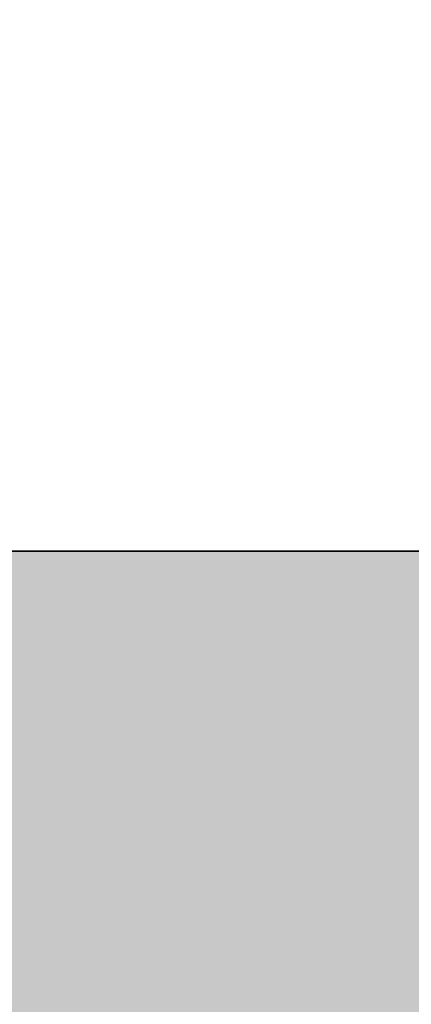
# Model space of a CAD drawing. Units: inches. Extents: x 2696 to 3240, y 1564 to 2310.
# Tile 58 of 76: x 2916.85 to 2921.79, y 2179.88 to 2192.31. Entities that reach past the tile are written whole.
import ezdxf

# ---------------------------------------------------------------- set-up
doc = ezdxf.new("R2010")
doc.units = ezdxf.units.IN
for name, color, linetype, lineweight in [('A-ANNO-DIMS', 3, 'Continuous', 18), ('A-WALL', 7, 'Continuous', 35), ('A-WALL-PATT', 9, 'Continuous', 13)]:
    doc.layers.add(name, color=color, linetype=linetype, lineweight=lineweight)
doc.styles.add('TIMES NEW', font='times.ttf')
doc.dimstyles.new('Siddhuu', dxfattribs={"dimtxt": 6, "dimasz": 2.5, "dimexe": 1.25, "dimexo": 0.625, "dimtad": 1, "dimdec": 1, "dimlunit": 4, "dimtxsty": 'TIMES NEW', "dimcen": 2.5, "dimclrd": 256, "dimclre": 1, "dimclrt": 7, "dimadec": 0, "dimazin": 0, "dimtfac": 1, "dimtdec": 1, "dimtmove": 0, "dimatfit": 3, "dimfxl": 1, "dimtolj": 1, "dimlwd": -1, "dimarcsym": 0})

# ---------------------------------------------------------------- blocks, each defined once
blk = doc.blocks.new('*D59')
at = {"layer": 'A-ANNO-DIMS', "color": 1, "lineweight": -2, "transparency": 16777216}
for p, q in [((2884.709, 1740.826), (2884.709, 2298.451)), ((2956.709, 1740.826), (2956.709, 2298.451))]:
    blk.add_line(p, q, dxfattribs=at)
at = {"layer": 'A-ANNO-DIMS', "transparency": 16777216}
blk.add_line((2887.209, 2297.201), (2954.209, 2297.201), dxfattribs=at)
for points in [[(2887.209, 2297.618), (2887.209, 2296.784), (2884.709, 2297.201)], [(2954.209, 2297.618), (2954.209, 2296.784), (2956.709, 2297.201)]]:
    blk.add_solid(points, dxfattribs=at)
at = {"layer": 'Defpoints', "color": 0, "transparency": 16777216}
for p in [(2956.709, 2297.201), (2884.709, 1740.201), (2956.709, 1740.201)]:
    blk.add_point(p, dxfattribs=at)
at = {"layer": 'A-ANNO-DIMS', "color": 7, "transparency": 16777216, "insert": (2920.709, 2300.878), "char_height": 6, "attachment_point": 5, "style": 'TIMES NEW'}
blk.add_mtext('\\A1;6\'-0"', dxfattribs=at)
blk = doc.blocks.new('*D64')
at = {"layer": 'A-ANNO-DIMS', "color": 1, "lineweight": -2, "transparency": 16777216}
for p, q in [((3073.084, 2206.701), (2709.361, 2206.701)), ((3068.584, 1989.201), (2709.361, 1989.201))]:
    blk.add_line(p, q, dxfattribs=at)
at = {"layer": 'A-ANNO-DIMS', "transparency": 16777216}
blk.add_line((2710.611, 1991.701), (2710.611, 2204.201), dxfattribs=at)
for points in [[(2710.195, 2204.201), (2711.028, 2204.201), (2710.611, 2206.701)], [(2710.195, 1991.701), (2711.028, 1991.701), (2710.611, 1989.201)]]:
    blk.add_solid(points, dxfattribs=at)
at = {"layer": 'Defpoints', "color": 0, "transparency": 16777216}
for p in [(2710.611, 2206.701), (3073.709, 2206.701), (3069.209, 1989.201)]:
    blk.add_point(p, dxfattribs=at)
at = {"layer": 'A-ANNO-DIMS', "color": 7, "transparency": 16777216, "insert": (2706.85, 2097.951), "char_height": 6, "attachment_point": 5, "rotation": 90, "style": 'TIMES NEW'}
blk.add_mtext('\\A1;18\'-1 1/2"', dxfattribs=at)

msp = doc.modelspace()

# ---------------------------------------------------------------- hatches: boundary and pattern name
at = {"layer": 'A-WALL-PATT', "transparency": 33554556}
h = msp.add_hatch(color=256, dxfattribs=at)
h.dxf.hatch_style = 1
h.paths.add_polyline_path([(2879.111, 2253.201), (2905.91, 2253.201), (2905.91, 2262.201), (2841.889, 2262.201), (2841.889, 2253.201), (2870.111, 2253.201), (2870.111, 2176.601), (2965.709, 2176.601), (2965.709, 2206.701), (2973.583, 2206.701), (2973.583, 2215.701), (2965.709, 2215.701), (2965.709, 2262.201), (2929.91, 2262.201), (2929.91, 2253.201), (2956.709, 2253.201), (2956.709, 2185.601), (2879.111, 2185.601)])
h.paths.add_polyline_path([(2782.834, 2262.201), (2745.611, 2262.201), (2745.611, 2228.729), (2754.611, 2228.729), (2754.611, 2253.201), (2782.834, 2253.201)])
h.paths.add_polyline_path([(2754.611, 2136.201), (2965.709, 2136.201), (2965.709, 2145.201), (2879.111, 2145.201), (2879.111, 2147.074), (2877.34, 2147.074), (2870.111, 2147.074), (2870.111, 2145.201), (2754.611, 2145.201), (2754.611, 2169.674), (2745.611, 2169.674), (2745.611, 2000.201), (2754.611, 2000.201), (2754.611, 2019.201), (2849.083, 2019.201), (2849.083, 2023.701), (2841.209, 2023.701), (2841.209, 2051.827), (2836.709, 2051.827), (2836.709, 2023.701), (2754.611, 2023.701), (2754.611, 2091.201), (2836.709, 2091.201), (2836.709, 2087.827), (2841.209, 2087.827), (2841.209, 2095.701), (2754.611, 2095.701)])
h.paths.add_polyline_path([(2965.709, 2136.201), (2956.709, 2136.201), (2956.709, 2023.701), (2885.083, 2023.701), (2885.083, 2019.201), (2956.709, 2019.201), (2956.709, 1950.575), (2965.709, 1950.575), (2965.709, 1980.201), (2973.583, 1980.201), (2973.583, 1989.201), (2965.709, 1989.201)])
h.paths.add_polyline_path([(2754.611, 1906.701), (2880.209, 1906.701), (2884.709, 1906.701), (2956.709, 1906.701), (2956.709, 1792.701), (2944.709, 1792.701), (2944.709, 1783.701), (2956.709, 1783.701), (2956.709, 1740.201), (2884.709, 1740.201), (2884.709, 1783.701), (2896.709, 1783.701), (2896.709, 1792.701), (2884.709, 1792.701), (2884.709, 1846.701), (2880.209, 1846.701), (2880.209, 1740.201), (2754.611, 1740.201), (2754.611, 1777.201), (2745.611, 1777.201), (2745.611, 1692.701), (2754.611, 1692.701), (2754.611, 1731.201), (2956.709, 1731.201), (2956.709, 1723.327), (2965.709, 1723.327), (2965.709, 1884.201), (2973.583, 1884.201), (2973.583, 1893.201), (2965.709, 1893.201), (2965.709, 1914.575), (2956.709, 1914.575), (2956.709, 1911.201), (2754.611, 1911.201), (2754.611, 1930.201), (2745.611, 1930.201), (2745.611, 1817.201), (2754.611, 1817.201), (2754.611, 1854.201), (2826.611, 1854.201), (2826.611, 1868.827), (2822.111, 1868.827), (2822.111, 1858.701), (2754.611, 1858.701)])
h.paths.add_polyline_path([(2965.709, 1656.201), (3008.237, 1656.201), (3008.237, 1665.201), (2965.709, 1665.201), (2965.709, 1693.327), (2956.709, 1693.327), (2956.709, 1686.201), (2934.583, 1686.201), (2934.583, 1681.701), (2956.709, 1681.701), (2956.709, 1614.201), (2896.709, 1614.201), (2896.709, 1681.701), (2904.583, 1681.701), (2904.583, 1686.201), (2892.209, 1686.201), (2892.209, 1614.201), (2858.41, 1614.201), (2858.41, 1605.201), (2965.709, 1605.201)])
h.paths.add_polyline_path([(2788.41, 1614.201), (2754.611, 1614.201), (2754.611, 1652.701), (2745.611, 1652.701), (2745.611, 1605.201), (2788.41, 1605.201)])
h.paths.add_polyline_path([(3199.611, 1633.048), (3190.611, 1633.048), (3190.611, 1614.201), (3082.611, 1614.201), (3082.611, 1665.201), (3070.237, 1665.201), (3070.237, 1656.201), (3078.111, 1656.201), (3078.111, 1605.201), (3199.611, 1605.201)])
h.paths.add_polyline_path([(3199.611, 1702.048), (3190.611, 1702.048), (3190.611, 1699.701), (3106.611, 1699.701), (3106.611, 1747.701), (3190.611, 1747.701), (3190.611, 1752.201), (3082.611, 1752.201), (3082.611, 1760.075), (3078.111, 1760.075), (3078.111, 1747.701), (3102.111, 1747.701), (3102.111, 1699.701), (3078.111, 1699.701), (3078.111, 1695.201), (3190.611, 1695.201), (3190.611, 1676.355), (3199.611, 1676.355)])
h.paths.add_polyline_path([(3199.611, 1783.201), (3190.611, 1783.201), (3190.611, 1745.355), (3199.611, 1745.355)])
h.paths.add_polyline_path([(3082.611, 1884.201), (3190.611, 1884.201), (3190.611, 1853.201), (3199.611, 1853.201), (3199.611, 1901.701), (3190.611, 1901.701), (3190.611, 1893.201), (3005.583, 1893.201), (3005.583, 1891.281), (3005.583, 1884.201), (3078.111, 1884.201), (3078.111, 1792.075), (3082.611, 1792.075)])
h.paths.add_polyline_path([(3199.611, 1994.701), (3190.611, 1994.701), (3190.611, 1989.201), (3073.709, 1989.201), (3073.709, 2034.201), (3069.209, 2034.201), (3069.209, 1989.201), (3005.583, 1989.201), (3005.583, 1980.201), (3190.611, 1980.201), (3190.611, 1971.701), (3199.611, 1971.701)])
h.paths.add_polyline_path([(3199.611, 2155.201), (3190.611, 2155.201), (3190.611, 2064.701), (3199.611, 2064.701)])
h.paths.add_polyline_path([(3190.611, 2074.701), (3106.611, 2074.701), (3106.611, 2122.701), (3190.611, 2122.701), (3190.611, 2127.201), (3082.709, 2127.201), (3082.709, 2135.075), (3073.709, 2135.075), (3073.709, 2122.701), (3102.111, 2122.701), (3102.111, 2074.701), (3069.209, 2074.701), (3069.209, 2070.201), (3190.611, 2070.201)])
h.paths.add_polyline_path([(3082.709, 2253.201), (3190.611, 2253.201), (3190.611, 2225.201), (3199.611, 2225.201), (3199.611, 2262.201), (3073.709, 2262.201), (3073.709, 2215.701), (3035.583, 2215.701), (3035.583, 2206.701), (3073.709, 2206.701), (3073.709, 2171.075), (3082.709, 2171.075)])

# ---------------------------------------------------------------- linework, layer by layer
at = {"layer": 'A-WALL'}
msp.add_line((2879.111, 2185.601), (2956.709, 2185.601), dxfattribs=at)

# ---------------------------------------------------------------- dimensions: what is measured, and where the dimension line sits
at = {"layer": 'A-ANNO-DIMS'}
dim = msp.add_linear_dim(base=(2956.709, 2297.201), p1=(2884.709, 1740.201), p2=(2956.709, 1740.201), dimstyle='Siddhuu', override={"dimdec": 1, "dimlfac": 1, "dimrnd": 0, "dimzin": 1, "dimdsep": 46, "dimlunit": 4, "dimfrac": 2}, dxfattribs=at)
dim.commit()
dim.dimension.update_dxf_attribs({"geometry": '*D59', "text_midpoint": (2920.709, 2300.878)})
dim = msp.add_linear_dim(base=(2710.611, 2206.701), p1=(3069.209, 1989.201), p2=(3073.709, 2206.701), angle=90, dimstyle='Siddhuu', override={"dimdec": 1, "dimlfac": 1, "dimrnd": 0, "dimzin": 1, "dimdsep": 46, "dimlunit": 4, "dimfrac": 2}, dxfattribs=at)
dim.commit()
dim.dimension.update_dxf_attribs({"geometry": '*D64', "text_midpoint": (2706.85, 2097.951)})

doc.saveas('drawing.dxf')
